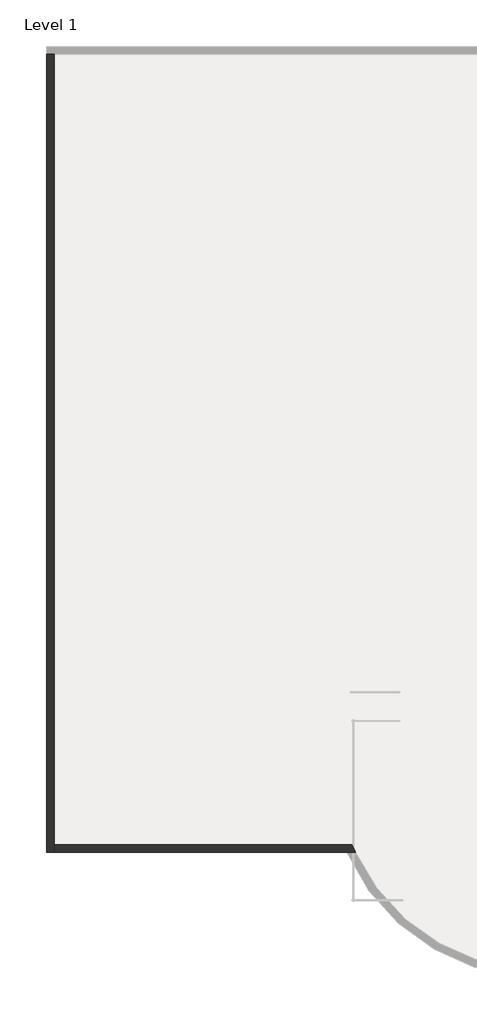
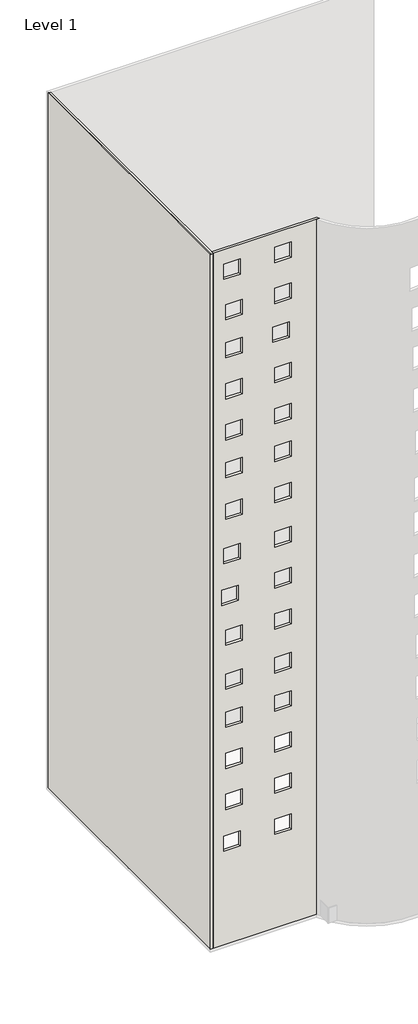
# One storey, part 1 of 3: 2 walls.
"""IFC4 building model written with IfcOpenShell, lengths in millimetres."""

from ifc_helpers import new_model, si_unit, frame, origin, place, context, project, spatial, polyline, circle_curve, faceted_brep, element, save
from ifc_brep_helpers import plane_surface, revolved_surface, advanced_brep

model = new_model("IFC4")

# Units and contexts
model_context = context("Model", 3, world=origin())
ifc_project = project(units=[si_unit("LENGTHUNIT", "METRE", prefix="MILLI")], contexts=[model_context])

# Site, building, storey
site = spatial("IfcSite", under=ifc_project)
building = spatial("IfcBuilding", under=site)
storey = spatial("IfcBuildingStorey", under=building, Name="Level 1", Elevation=0.0)

# Walls
placement = place(None, origin())
element("IfcWall", 1, ObjectType="Generic - 8\"", at=placement, inside=storey, context=model_context, shape_type="Brep", body=[
    faceted_brep([(-16607.9505427, 7156.3191779, 0.0), (-16607.9505427, -14078.0808221, 0.0), (-16607.9505427, -14078.0808221, 55473.6), (-16607.9505427, 7156.3191779, 55473.6), (-16404.7505427, 7156.3191779, 0.0), (-16404.7505427, 7156.3191779, 55473.6), (-16404.7505427, -13874.8808221, 55473.6), (-16404.7505427, -14078.0808221, 55473.6), (-16404.7505427, -14078.0808221, 0.0), (-16404.7505427, -13874.8808221, 0.0), (-16556.2150607, 7156.3191779, 55473.6), (-16556.2150607, -14078.0808221, 55473.6)], [[[0, 1, 2, 3]], [[4, 5, 6, 7, 8, 9]], [[1, 0, 4, 9, 8]], [[0, 3, 10, 5, 4]], [[2, 1, 8, 7, 11]], [[3, 2, 11, 10]], [[11, 7, 6, 5, 10]]]),
])
element("IfcWall", 2, ObjectType="Generic - 8\"", at=placement, inside=storey, context=model_context, shape_type="AdvancedBrep", body=[
    advanced_brep(
    [(-16404.7505427, -14078.0808221, 0.0), (-8605.1750786, -14078.0808221, 0.0), (-8381.8075047, -14078.0808221, 0.0), (-8381.8075047, -14078.0808221, 55473.6), (-8605.1750786, -14078.0808221, 55473.6), (-16404.7505427, -14078.0808221, 55473.6), (-15591.9505427, -14078.0808221, 54330.6), (-14372.7505427, -14078.0808221, 54330.6), (-14372.7505427, -14078.0808221, 53111.4), (-15591.9505427, -14078.0808221, 53111.4), (-11739.2382271, -14078.0808221, 54330.6), (-10520.0382271, -14078.0808221, 54330.6), (-10520.0382271, -14078.0808221, 53111.4), (-11739.2382271, -14078.0808221, 53111.4), (-15439.5505427, -14078.0808221, 51054.0), (-14220.3505427, -14078.0808221, 51054.0), (-14220.3505427, -14078.0808221, 49834.8), (-15439.5505427, -14078.0808221, 49834.8), (-11739.2382271, -14078.0808221, 51054.0), (-10520.0382271, -14078.0808221, 51054.0), (-10520.0382271, -14078.0808221, 49834.8), (-11739.2382271, -14078.0808221, 49834.8), (-15439.5505427, -14078.0808221, 48006.0), (-14220.3505427, -14078.0808221, 48006.0), (-14220.3505427, -14078.0808221, 46786.8), (-15439.5505427, -14078.0808221, 46786.8), (-11891.6382271, -14078.0808221, 48006.0), (-10672.4382271, -14078.0808221, 48006.0), (-10672.4382271, -14078.0808221, 46786.8), (-11891.6382271, -14078.0808221, 46786.8), (-15439.5505427, -14078.0808221, 44729.4), (-14220.3505427, -14078.0808221, 44729.4), (-14220.3505427, -14078.0808221, 43510.2), (-15439.5505427, -14078.0808221, 43510.2), (-11739.2382271, -14078.0808221, 44729.4), (-10520.0382271, -14078.0808221, 44729.4), (-10520.0382271, -14078.0808221, 43510.2), (-11739.2382271, -14078.0808221, 43510.2), (-15439.5505427, -14078.0808221, 41452.8), (-14220.3505427, -14078.0808221, 41452.8), (-14220.3505427, -14078.0808221, 40233.6), (-15439.5505427, -14078.0808221, 40233.6), (-11739.2382271, -14078.0808221, 41452.8), (-10520.0382271, -14078.0808221, 41452.8), (-10520.0382271, -14078.0808221, 40233.6), (-11739.2382271, -14078.0808221, 40233.6), (-15439.5505427, -14078.0808221, 38436.7791335), (-14220.3505427, -14078.0808221, 38436.7791335), (-14220.3505427, -14078.0808221, 37217.5791335), (-15439.5505427, -14078.0808221, 37217.5791335), (-11739.2382271, -14078.0808221, 38440.5564743), (-10520.0382271, -14078.0808221, 38440.5564743), (-10520.0382271, -14078.0808221, 37221.3564743), (-11739.2382271, -14078.0808221, 37221.3564743), (-15439.5505427, -14078.0808221, 35116.3338162), (-14220.3505427, -14078.0808221, 35116.3338162), (-14220.3505427, -14078.0808221, 33897.1338162), (-15439.5505427, -14078.0808221, 33897.1338162), (-11739.2382271, -14078.0808221, 35146.4998834), (-10520.0382271, -14078.0808221, 35146.4998834), (-10520.0382271, -14078.0808221, 33927.2998834), (-11739.2382271, -14078.0808221, 33927.2998834), (-15591.9505427, -14078.0808221, 31623.0), (-14372.7505427, -14078.0808221, 31623.0), (-14372.7505427, -14078.0808221, 30403.8), (-15591.9505427, -14078.0808221, 30403.8), (-11739.2382271, -14078.0808221, 31623.0), (-10520.0382271, -14078.0808221, 31623.0), (-10520.0382271, -14078.0808221, 30403.8), (-11739.2382271, -14078.0808221, 30403.8), (-15744.3505427, -14078.0808221, 28346.4), (-14525.1505427, -14078.0808221, 28346.4), (-14525.1505427, -14078.0808221, 27127.2), (-15744.3505427, -14078.0808221, 27127.2), (-11739.2382271, -14078.0808221, 28346.4), (-10520.0382271, -14078.0808221, 28346.4), (-10520.0382271, -14078.0808221, 27127.2), (-11739.2382271, -14078.0808221, 27127.2), (-15439.5505427, -14078.0808221, 25069.8), (-14220.3505427, -14078.0808221, 25069.8), (-14220.3505427, -14078.0808221, 23850.6), (-15439.5505427, -14078.0808221, 23850.6), (-11739.2382271, -14078.0808221, 25069.8), (-10520.0382271, -14078.0808221, 25069.8), (-10520.0382271, -14078.0808221, 23850.6), (-11739.2382271, -14078.0808221, 23850.6), (-15439.5505427, -14078.0808221, 21564.6), (-14220.3505427, -14078.0808221, 21564.6), (-14220.3505427, -14078.0808221, 20345.4), (-15439.5505427, -14078.0808221, 20345.4), (-11739.2382271, -14078.0808221, 21564.6), (-10520.0382271, -14078.0808221, 21564.6), (-10520.0382271, -14078.0808221, 20345.4), (-11739.2382271, -14078.0808221, 20345.4), (-11739.2382271, -14078.0808221, 18516.6), (-10520.0382271, -14078.0808221, 18516.6), (-10520.0382271, -14078.0808221, 17297.4), (-11739.2382271, -14078.0808221, 17297.4), (-15439.5505427, -14078.0808221, 18516.6), (-14220.3505427, -14078.0808221, 18516.6), (-14220.3505427, -14078.0808221, 17297.4), (-15439.5505427, -14078.0808221, 17297.4), (-11739.2382271, -14078.0808221, 15240.0), (-10520.0382271, -14078.0808221, 15240.0), (-10520.0382271, -14078.0808221, 14020.8), (-11739.2382271, -14078.0808221, 14020.8), (-15439.5505427, -14078.0808221, 15240.0), (-14220.3505427, -14078.0808221, 15240.0), (-14220.3505427, -14078.0808221, 14020.8), (-15439.5505427, -14078.0808221, 14020.8), (-11739.2382271, -14078.0808221, 11963.4), (-10520.0382271, -14078.0808221, 11963.4), (-10520.0382271, -14078.0808221, 10744.2), (-11739.2382271, -14078.0808221, 10744.2), (-15439.5505427, -14078.0808221, 11963.4), (-14220.3505427, -14078.0808221, 11963.4), (-14220.3505427, -14078.0808221, 10744.2), (-15439.5505427, -14078.0808221, 10744.2), (-15591.9505427, -14078.0808221, 8686.8), (-14372.7505427, -14078.0808221, 8686.8), (-14372.7505427, -14078.0808221, 7467.6), (-15591.9505427, -14078.0808221, 7467.6), (-11739.2382271, -14078.0808221, 8686.8), (-10520.0382271, -14078.0808221, 8686.8), (-10520.0382271, -14078.0808221, 7467.6), (-11739.2382271, -14078.0808221, 7467.6), (-16404.7505427, -13874.8808221, 0.0), (-16404.7505427, -13874.8808221, 55473.6), (-8471.6205396, -13874.8808221, 55473.6), (-8471.6205396, -13874.8808221, 0.0), (-15591.9505427, -13874.8808221, 54330.6), (-15591.9505427, -13874.8808221, 53111.4), (-14372.7505427, -13874.8808221, 53111.4), (-14372.7505427, -13874.8808221, 54330.6), (-11739.2382271, -13874.8808221, 54330.6), (-11739.2382271, -13874.8808221, 53111.4), (-10520.0382271, -13874.8808221, 53111.4), (-10520.0382271, -13874.8808221, 54330.6), (-15439.5505427, -13874.8808221, 51054.0), (-15439.5505427, -13874.8808221, 49834.8), (-14220.3505427, -13874.8808221, 49834.8), (-14220.3505427, -13874.8808221, 51054.0), (-11739.2382271, -13874.8808221, 51054.0), (-11739.2382271, -13874.8808221, 49834.8), (-10520.0382271, -13874.8808221, 49834.8), (-10520.0382271, -13874.8808221, 51054.0), (-15439.5505427, -13874.8808221, 48006.0), (-15439.5505427, -13874.8808221, 46786.8), (-14220.3505427, -13874.8808221, 46786.8), (-14220.3505427, -13874.8808221, 48006.0), (-11891.6382271, -13874.8808221, 48006.0), (-11891.6382271, -13874.8808221, 46786.8), (-10672.4382271, -13874.8808221, 46786.8), (-10672.4382271, -13874.8808221, 48006.0), (-15439.5505427, -13874.8808221, 44729.4), (-15439.5505427, -13874.8808221, 43510.2), (-14220.3505427, -13874.8808221, 43510.2), (-14220.3505427, -13874.8808221, 44729.4), (-11739.2382271, -13874.8808221, 44729.4), (-11739.2382271, -13874.8808221, 43510.2), (-10520.0382271, -13874.8808221, 43510.2), (-10520.0382271, -13874.8808221, 44729.4), (-15439.5505427, -13874.8808221, 41452.8), (-15439.5505427, -13874.8808221, 40233.6), (-14220.3505427, -13874.8808221, 40233.6), (-14220.3505427, -13874.8808221, 41452.8), (-11739.2382271, -13874.8808221, 41452.8), (-11739.2382271, -13874.8808221, 40233.6), (-10520.0382271, -13874.8808221, 40233.6), (-10520.0382271, -13874.8808221, 41452.8), (-15439.5505427, -13874.8808221, 38436.7791335), (-15439.5505427, -13874.8808221, 37217.5791335), (-14220.3505427, -13874.8808221, 37217.5791335), (-14220.3505427, -13874.8808221, 38436.7791335), (-11739.2382271, -13874.8808221, 38440.5564743), (-11739.2382271, -13874.8808221, 37221.3564743), (-10520.0382271, -13874.8808221, 37221.3564743), (-10520.0382271, -13874.8808221, 38440.5564743), (-15439.5505427, -13874.8808221, 35116.3338162), (-15439.5505427, -13874.8808221, 33897.1338162), (-14220.3505427, -13874.8808221, 33897.1338162), (-14220.3505427, -13874.8808221, 35116.3338162), (-11739.2382271, -13874.8808221, 35146.4998834), (-11739.2382271, -13874.8808221, 33927.2998834), (-10520.0382271, -13874.8808221, 33927.2998834), (-10520.0382271, -13874.8808221, 35146.4998834), (-15591.9505427, -13874.8808221, 31623.0), (-15591.9505427, -13874.8808221, 30403.8), (-14372.7505427, -13874.8808221, 30403.8), (-14372.7505427, -13874.8808221, 31623.0), (-11739.2382271, -13874.8808221, 31623.0), (-11739.2382271, -13874.8808221, 30403.8), (-10520.0382271, -13874.8808221, 30403.8), (-10520.0382271, -13874.8808221, 31623.0), (-15744.3505427, -13874.8808221, 28346.4), (-15744.3505427, -13874.8808221, 27127.2), (-14525.1505427, -13874.8808221, 27127.2), (-14525.1505427, -13874.8808221, 28346.4), (-11739.2382271, -13874.8808221, 28346.4), (-11739.2382271, -13874.8808221, 27127.2), (-10520.0382271, -13874.8808221, 27127.2), (-10520.0382271, -13874.8808221, 28346.4), (-15439.5505427, -13874.8808221, 25069.8), (-15439.5505427, -13874.8808221, 23850.6), (-14220.3505427, -13874.8808221, 23850.6), (-14220.3505427, -13874.8808221, 25069.8), (-11739.2382271, -13874.8808221, 25069.8), (-11739.2382271, -13874.8808221, 23850.6), (-10520.0382271, -13874.8808221, 23850.6), (-10520.0382271, -13874.8808221, 25069.8), (-15439.5505427, -13874.8808221, 21564.6), (-15439.5505427, -13874.8808221, 20345.4), (-14220.3505427, -13874.8808221, 20345.4), (-14220.3505427, -13874.8808221, 21564.6), (-11739.2382271, -13874.8808221, 21564.6), (-11739.2382271, -13874.8808221, 20345.4), (-10520.0382271, -13874.8808221, 20345.4), (-10520.0382271, -13874.8808221, 21564.6), (-11739.2382271, -13874.8808221, 18516.6), (-11739.2382271, -13874.8808221, 17297.4), (-10520.0382271, -13874.8808221, 17297.4), (-10520.0382271, -13874.8808221, 18516.6), (-15439.5505427, -13874.8808221, 18516.6), (-15439.5505427, -13874.8808221, 17297.4), (-14220.3505427, -13874.8808221, 17297.4), (-14220.3505427, -13874.8808221, 18516.6), (-11739.2382271, -13874.8808221, 15240.0), (-11739.2382271, -13874.8808221, 14020.8), (-10520.0382271, -13874.8808221, 14020.8), (-10520.0382271, -13874.8808221, 15240.0), (-15439.5505427, -13874.8808221, 15240.0), (-15439.5505427, -13874.8808221, 14020.8), (-14220.3505427, -13874.8808221, 14020.8), (-14220.3505427, -13874.8808221, 15240.0), (-11739.2382271, -13874.8808221, 11963.4), (-11739.2382271, -13874.8808221, 10744.2), (-10520.0382271, -13874.8808221, 10744.2), (-10520.0382271, -13874.8808221, 11963.4), (-15439.5505427, -13874.8808221, 11963.4), (-15439.5505427, -13874.8808221, 10744.2), (-14220.3505427, -13874.8808221, 10744.2), (-14220.3505427, -13874.8808221, 11963.4), (-15591.9505427, -13874.8808221, 8686.8), (-15591.9505427, -13874.8808221, 7467.6), (-14372.7505427, -13874.8808221, 7467.6), (-14372.7505427, -13874.8808221, 8686.8), (-11739.2382271, -13874.8808221, 8686.8), (-11739.2382271, -13874.8808221, 7467.6), (-10520.0382271, -13874.8808221, 7467.6), (-10520.0382271, -13874.8808221, 8686.8)],
    [
        (0, 1),
        (1, 2),
        (2, 3),
        (3, 4),
        (4, 5),
        (5, 0),
        (6, 7),
        (7, 8),
        (8, 9),
        (9, 6),
        (10, 11),
        (11, 12),
        (12, 13),
        (13, 10),
        (14, 15),
        (15, 16),
        (16, 17),
        (17, 14),
        (18, 19),
        (19, 20),
        (20, 21),
        (21, 18),
        (22, 23),
        (23, 24),
        (24, 25),
        (25, 22),
        (26, 27),
        (27, 28),
        (28, 29),
        (29, 26),
        (30, 31),
        (31, 32),
        (32, 33),
        (33, 30),
        (34, 35),
        (35, 36),
        (36, 37),
        (37, 34),
        (38, 39),
        (39, 40),
        (40, 41),
        (41, 38),
        (42, 43),
        (43, 44),
        (44, 45),
        (45, 42),
        (46, 47),
        (47, 48),
        (48, 49),
        (49, 46),
        (50, 51),
        (51, 52),
        (52, 53),
        (53, 50),
        (54, 55),
        (55, 56),
        (56, 57),
        (57, 54),
        (58, 59),
        (59, 60),
        (60, 61),
        (61, 58),
        (62, 63),
        (63, 64),
        (64, 65),
        (65, 62),
        (66, 67),
        (67, 68),
        (68, 69),
        (69, 66),
        (70, 71),
        (71, 72),
        (72, 73),
        (73, 70),
        (74, 75),
        (75, 76),
        (76, 77),
        (77, 74),
        (78, 79),
        (79, 80),
        (80, 81),
        (81, 78),
        (82, 83),
        (83, 84),
        (84, 85),
        (85, 82),
        (86, 87),
        (87, 88),
        (88, 89),
        (89, 86),
        (90, 91),
        (91, 92),
        (92, 93),
        (93, 90),
        (94, 95),
        (95, 96),
        (96, 97),
        (97, 94),
        (98, 99),
        (99, 100),
        (100, 101),
        (101, 98),
        (102, 103),
        (103, 104),
        (104, 105),
        (105, 102),
        (106, 107),
        (107, 108),
        (108, 109),
        (109, 106),
        (110, 111),
        (111, 112),
        (112, 113),
        (113, 110),
        (114, 115),
        (115, 116),
        (116, 117),
        (117, 114),
        (118, 119),
        (119, 120),
        (120, 121),
        (121, 118),
        (122, 123),
        (123, 124),
        (124, 125),
        (125, 122),
        (126, 127),
        (127, 128),
        (128, 129),
        (129, 126),
        (130, 131),
        (131, 132),
        (132, 133),
        (133, 130),
        (134, 135),
        (135, 136),
        (136, 137),
        (137, 134),
        (138, 139),
        (139, 140),
        (140, 141),
        (141, 138),
        (142, 143),
        (143, 144),
        (144, 145),
        (145, 142),
        (146, 147),
        (147, 148),
        (148, 149),
        (149, 146),
        (150, 151),
        (151, 152),
        (152, 153),
        (153, 150),
        (154, 155),
        (155, 156),
        (156, 157),
        (157, 154),
        (158, 159),
        (159, 160),
        (160, 161),
        (161, 158),
        (162, 163),
        (163, 164),
        (164, 165),
        (165, 162),
        (166, 167),
        (167, 168),
        (168, 169),
        (169, 166),
        (170, 171),
        (171, 172),
        (172, 173),
        (173, 170),
        (174, 175),
        (175, 176),
        (176, 177),
        (177, 174),
        (178, 179),
        (179, 180),
        (180, 181),
        (181, 178),
        (182, 183),
        (183, 184),
        (184, 185),
        (185, 182),
        (186, 187),
        (187, 188),
        (188, 189),
        (189, 186),
        (190, 191),
        (191, 192),
        (192, 193),
        (193, 190),
        (194, 195),
        (195, 196),
        (196, 197),
        (197, 194),
        (198, 199),
        (199, 200),
        (200, 201),
        (201, 198),
        (202, 203),
        (203, 204),
        (204, 205),
        (205, 202),
        (206, 207),
        (207, 208),
        (208, 209),
        (209, 206),
        (210, 211),
        (211, 212),
        (212, 213),
        (213, 210),
        (214, 215),
        (215, 216),
        (216, 217),
        (217, 214),
        (218, 219),
        (219, 220),
        (220, 221),
        (221, 218),
        (222, 223),
        (223, 224),
        (224, 225),
        (225, 222),
        (226, 227),
        (227, 228),
        (228, 229),
        (229, 226),
        (230, 231),
        (231, 232),
        (232, 233),
        (233, 230),
        (234, 235),
        (235, 236),
        (236, 237),
        (237, 234),
        (238, 239),
        (239, 240),
        (240, 241),
        (241, 238),
        (242, 243),
        (243, 244),
        (244, 245),
        (245, 242),
        (246, 247),
        (247, 248),
        (248, 249),
        (249, 246),
        (0, 126),
        (129, 2, circle_curve(frame((-3476.1505427, -11788.3650223, 0.0), z_axis=(0.0, 0.0, 1.0), x_axis=(1.0, 0.0, 0.0)), 5413.7111737)),
        (5, 127),
        (128, 3, circle_curve(frame((-3476.1505427, -11788.3650223, 55473.6), z_axis=(0.0, 0.0, 1.0), x_axis=(1.0, 0.0, 0.0)), 5413.7111737)),
        (130, 6),
        (9, 131),
        (8, 132),
        (7, 133),
        (134, 10),
        (13, 135),
        (12, 136),
        (11, 137),
        (138, 14),
        (17, 139),
        (16, 140),
        (15, 141),
        (142, 18),
        (21, 143),
        (20, 144),
        (19, 145),
        (146, 22),
        (25, 147),
        (24, 148),
        (23, 149),
        (150, 26),
        (29, 151),
        (28, 152),
        (27, 153),
        (154, 30),
        (33, 155),
        (32, 156),
        (31, 157),
        (158, 34),
        (37, 159),
        (36, 160),
        (35, 161),
        (162, 38),
        (41, 163),
        (40, 164),
        (39, 165),
        (166, 42),
        (45, 167),
        (44, 168),
        (43, 169),
        (170, 46),
        (49, 171),
        (48, 172),
        (47, 173),
        (174, 50),
        (53, 175),
        (52, 176),
        (51, 177),
        (178, 54),
        (57, 179),
        (56, 180),
        (55, 181),
        (182, 58),
        (61, 183),
        (60, 184),
        (59, 185),
        (186, 62),
        (65, 187),
        (64, 188),
        (63, 189),
        (190, 66),
        (69, 191),
        (68, 192),
        (67, 193),
        (194, 70),
        (73, 195),
        (72, 196),
        (71, 197),
        (198, 74),
        (77, 199),
        (76, 200),
        (75, 201),
        (202, 78),
        (81, 203),
        (80, 204),
        (79, 205),
        (206, 82),
        (85, 207),
        (84, 208),
        (83, 209),
        (210, 86),
        (89, 211),
        (88, 212),
        (87, 213),
        (214, 90),
        (93, 215),
        (92, 216),
        (91, 217),
        (218, 94),
        (97, 219),
        (96, 220),
        (95, 221),
        (222, 98),
        (101, 223),
        (100, 224),
        (99, 225),
        (226, 102),
        (105, 227),
        (104, 228),
        (103, 229),
        (230, 106),
        (109, 231),
        (108, 232),
        (107, 233),
        (234, 110),
        (113, 235),
        (112, 236),
        (111, 237),
        (238, 114),
        (117, 239),
        (116, 240),
        (115, 241),
        (242, 118),
        (121, 243),
        (120, 244),
        (119, 245),
        (246, 122),
        (125, 247),
        (124, 248),
        (123, 249),
    ],
    [
        plane_surface(frame((-16506.3505427, -14078.0808221, 0.0), z_axis=(0.0, -1.0, 0.0), x_axis=(1.0, 0.0, 0.0))),
        plane_surface(frame((-16506.3505427, -13874.8808221, 0.0), z_axis=(0.0, 1.0, 0.0), x_axis=(-1.0, 0.0, 0.0))),
        plane_surface(frame((-16506.3505427, -14078.0808221, 0.0), z_axis=(0.0, 0.0, -1.0), x_axis=(0.0, 1.0, 0.0))),
        plane_surface(frame((-16404.7505427, 7359.5191779, 0.0), z_axis=(-1.0, 0.0, 0.0), x_axis=(0.0, 1.0, 0.0))),
        revolved_surface(polyline([(1937.5606309999994, -11788.3650223, 0.0), (1937.5606309999994, -11788.3650223, 55473.6)]), (-3476.1505427, -11788.3650223, 0.0), (0.0, 0.0, -1.0)),
        plane_surface(frame((-15591.9505427, -13874.8808221, 54330.6), z_axis=(1.0, 0.0, 0.0), x_axis=(0.0, -1.0, 0.0))),
        plane_surface(frame((-15591.9505427, -13874.8808221, 53111.4), z_axis=(0.0, 0.0, 1.0), x_axis=(0.0, -1.0, 0.0))),
        plane_surface(frame((-14372.7505427, -13874.8808221, 53111.4), z_axis=(-1.0, 0.0, 0.0), x_axis=(0.0, -1.0, 0.0))),
        plane_surface(frame((-14372.7505427, -13874.8808221, 54330.6), z_axis=(0.0, 0.0, -1.0), x_axis=(0.0, -1.0, 0.0))),
        plane_surface(frame((-11739.2382271, -13874.8808221, 54330.6), z_axis=(1.0, 0.0, 0.0), x_axis=(0.0, -1.0, 0.0))),
        plane_surface(frame((-11739.2382271, -13874.8808221, 53111.4), z_axis=(0.0, 0.0, 1.0), x_axis=(0.0, -1.0, 0.0))),
        plane_surface(frame((-10520.0382271, -13874.8808221, 53111.4), z_axis=(-1.0, 0.0, 0.0), x_axis=(0.0, -1.0, 0.0))),
        plane_surface(frame((-10520.0382271, -13874.8808221, 54330.6), z_axis=(0.0, 0.0, -1.0), x_axis=(0.0, -1.0, 0.0))),
        plane_surface(frame((-15439.5505427, -13874.8808221, 51054.0), z_axis=(1.0, 0.0, 0.0), x_axis=(0.0, -1.0, 0.0))),
        plane_surface(frame((-15439.5505427, -13874.8808221, 49834.8), z_axis=(0.0, 0.0, 1.0), x_axis=(0.0, -1.0, 0.0))),
        plane_surface(frame((-14220.3505427, -13874.8808221, 49834.8), z_axis=(-1.0, 0.0, 0.0), x_axis=(0.0, -1.0, 0.0))),
        plane_surface(frame((-14220.3505427, -13874.8808221, 51054.0), z_axis=(0.0, 0.0, -1.0), x_axis=(0.0, -1.0, 0.0))),
        plane_surface(frame((-11739.2382271, -13874.8808221, 51054.0), z_axis=(1.0, 0.0, 0.0), x_axis=(0.0, -1.0, 0.0))),
        plane_surface(frame((-11739.2382271, -13874.8808221, 49834.8), z_axis=(0.0, 0.0, 1.0), x_axis=(0.0, -1.0, 0.0))),
        plane_surface(frame((-10520.0382271, -13874.8808221, 49834.8), z_axis=(-1.0, 0.0, 0.0), x_axis=(0.0, -1.0, 0.0))),
        plane_surface(frame((-10520.0382271, -13874.8808221, 51054.0), z_axis=(0.0, 0.0, -1.0), x_axis=(0.0, -1.0, 0.0))),
        plane_surface(frame((-15439.5505427, -13874.8808221, 48006.0), z_axis=(1.0, 0.0, 0.0), x_axis=(0.0, -1.0, 0.0))),
        plane_surface(frame((-15439.5505427, -13874.8808221, 46786.8), z_axis=(0.0, 0.0, 1.0), x_axis=(0.0, -1.0, 0.0))),
        plane_surface(frame((-14220.3505427, -13874.8808221, 46786.8), z_axis=(-1.0, 0.0, 0.0), x_axis=(0.0, -1.0, 0.0))),
        plane_surface(frame((-14220.3505427, -13874.8808221, 48006.0), z_axis=(0.0, 0.0, -1.0), x_axis=(0.0, -1.0, 0.0))),
        plane_surface(frame((-11891.6382271, -13874.8808221, 48006.0), z_axis=(1.0, 0.0, 0.0), x_axis=(0.0, -1.0, 0.0))),
        plane_surface(frame((-11891.6382271, -13874.8808221, 46786.8), z_axis=(0.0, 0.0, 1.0), x_axis=(0.0, -1.0, 0.0))),
        plane_surface(frame((-10672.4382271, -13874.8808221, 46786.8), z_axis=(-1.0, 0.0, 0.0), x_axis=(0.0, -1.0, 0.0))),
        plane_surface(frame((-10672.4382271, -13874.8808221, 48006.0), z_axis=(0.0, 0.0, -1.0), x_axis=(0.0, -1.0, 0.0))),
        plane_surface(frame((-15439.5505427, -13874.8808221, 44729.4), z_axis=(1.0, 0.0, 0.0), x_axis=(0.0, -1.0, 0.0))),
        plane_surface(frame((-15439.5505427, -13874.8808221, 43510.2), z_axis=(0.0, 0.0, 1.0), x_axis=(0.0, -1.0, 0.0))),
        plane_surface(frame((-14220.3505427, -13874.8808221, 43510.2), z_axis=(-1.0, 0.0, 0.0), x_axis=(0.0, -1.0, 0.0))),
        plane_surface(frame((-14220.3505427, -13874.8808221, 44729.4), z_axis=(0.0, 0.0, -1.0), x_axis=(0.0, -1.0, 0.0))),
        plane_surface(frame((-11739.2382271, -13874.8808221, 44729.4), z_axis=(1.0, 0.0, 0.0), x_axis=(0.0, -1.0, 0.0))),
        plane_surface(frame((-11739.2382271, -13874.8808221, 43510.2), z_axis=(0.0, 0.0, 1.0), x_axis=(0.0, -1.0, 0.0))),
        plane_surface(frame((-10520.0382271, -13874.8808221, 43510.2), z_axis=(-1.0, 0.0, 0.0), x_axis=(0.0, -1.0, 0.0))),
        plane_surface(frame((-10520.0382271, -13874.8808221, 44729.4), z_axis=(0.0, 0.0, -1.0), x_axis=(0.0, -1.0, 0.0))),
        plane_surface(frame((-15439.5505427, -13874.8808221, 41452.8), z_axis=(1.0, 0.0, 0.0), x_axis=(0.0, -1.0, 0.0))),
        plane_surface(frame((-15439.5505427, -13874.8808221, 40233.6), z_axis=(0.0, 0.0, 1.0), x_axis=(0.0, -1.0, 0.0))),
        plane_surface(frame((-14220.3505427, -13874.8808221, 40233.6), z_axis=(-1.0, 0.0, 0.0), x_axis=(0.0, -1.0, 0.0))),
        plane_surface(frame((-14220.3505427, -13874.8808221, 41452.8), z_axis=(0.0, 0.0, -1.0), x_axis=(0.0, -1.0, 0.0))),
        plane_surface(frame((-11739.2382271, -13874.8808221, 41452.8), z_axis=(1.0, 0.0, 0.0), x_axis=(0.0, -1.0, 0.0))),
        plane_surface(frame((-11739.2382271, -13874.8808221, 40233.6), z_axis=(0.0, 0.0, 1.0), x_axis=(0.0, -1.0, 0.0))),
        plane_surface(frame((-10520.0382271, -13874.8808221, 40233.6), z_axis=(-1.0, 0.0, 0.0), x_axis=(0.0, -1.0, 0.0))),
        plane_surface(frame((-10520.0382271, -13874.8808221, 41452.8), z_axis=(0.0, 0.0, -1.0), x_axis=(0.0, -1.0, 0.0))),
        plane_surface(frame((-15439.5505427, -13874.8808221, 38436.7791335), z_axis=(1.0, 0.0, 0.0), x_axis=(0.0, -1.0, 0.0))),
        plane_surface(frame((-15439.5505427, -13874.8808221, 37217.5791335), z_axis=(0.0, 0.0, 1.0), x_axis=(0.0, -1.0, 0.0))),
        plane_surface(frame((-14220.3505427, -13874.8808221, 37217.5791335), z_axis=(-1.0, 0.0, 0.0), x_axis=(0.0, -1.0, 0.0))),
        plane_surface(frame((-14220.3505427, -13874.8808221, 38436.7791335), z_axis=(0.0, 0.0, -1.0), x_axis=(0.0, -1.0, 0.0))),
        plane_surface(frame((-11739.2382271, -13874.8808221, 38440.5564743), z_axis=(1.0, 0.0, 0.0), x_axis=(0.0, -1.0, 0.0))),
        plane_surface(frame((-11739.2382271, -13874.8808221, 37221.3564743), z_axis=(0.0, 0.0, 1.0), x_axis=(0.0, -1.0, 0.0))),
        plane_surface(frame((-10520.0382271, -13874.8808221, 37221.3564743), z_axis=(-1.0, 0.0, 0.0), x_axis=(0.0, -1.0, 0.0))),
        plane_surface(frame((-10520.0382271, -13874.8808221, 38440.5564743), z_axis=(0.0, 0.0, -1.0), x_axis=(0.0, -1.0, 0.0))),
        plane_surface(frame((-15439.5505427, -13874.8808221, 35116.3338162), z_axis=(1.0, 0.0, 0.0), x_axis=(0.0, -1.0, 0.0))),
        plane_surface(frame((-15439.5505427, -13874.8808221, 33897.1338162), z_axis=(0.0, 0.0, 1.0), x_axis=(0.0, -1.0, 0.0))),
        plane_surface(frame((-14220.3505427, -13874.8808221, 33897.1338162), z_axis=(-1.0, 0.0, 0.0), x_axis=(0.0, -1.0, 0.0))),
        plane_surface(frame((-14220.3505427, -13874.8808221, 35116.3338162), z_axis=(0.0, 0.0, -1.0), x_axis=(0.0, -1.0, 0.0))),
        plane_surface(frame((-11739.2382271, -13874.8808221, 35146.4998834), z_axis=(1.0, 0.0, 0.0), x_axis=(0.0, -1.0, 0.0))),
        plane_surface(frame((-11739.2382271, -13874.8808221, 33927.2998834), z_axis=(0.0, 0.0, 1.0), x_axis=(0.0, -1.0, 0.0))),
        plane_surface(frame((-10520.0382271, -13874.8808221, 33927.2998834), z_axis=(-1.0, 0.0, 0.0), x_axis=(0.0, -1.0, 0.0))),
        plane_surface(frame((-10520.0382271, -13874.8808221, 35146.4998834), z_axis=(0.0, 0.0, -1.0), x_axis=(0.0, -1.0, 0.0))),
        plane_surface(frame((-15591.9505427, -13874.8808221, 31623.0), z_axis=(1.0, 0.0, 0.0), x_axis=(0.0, -1.0, 0.0))),
        plane_surface(frame((-15591.9505427, -13874.8808221, 30403.8), z_axis=(0.0, 0.0, 1.0), x_axis=(0.0, -1.0, 0.0))),
        plane_surface(frame((-14372.7505427, -13874.8808221, 30403.8), z_axis=(-1.0, 0.0, 0.0), x_axis=(0.0, -1.0, 0.0))),
        plane_surface(frame((-14372.7505427, -13874.8808221, 31623.0), z_axis=(0.0, 0.0, -1.0), x_axis=(0.0, -1.0, 0.0))),
        plane_surface(frame((-11739.2382271, -13874.8808221, 31623.0), z_axis=(1.0, 0.0, 0.0), x_axis=(0.0, -1.0, 0.0))),
        plane_surface(frame((-11739.2382271, -13874.8808221, 30403.8), z_axis=(0.0, 0.0, 1.0), x_axis=(0.0, -1.0, 0.0))),
        plane_surface(frame((-10520.0382271, -13874.8808221, 30403.8), z_axis=(-1.0, 0.0, 0.0), x_axis=(0.0, -1.0, 0.0))),
        plane_surface(frame((-10520.0382271, -13874.8808221, 31623.0), z_axis=(0.0, 0.0, -1.0), x_axis=(0.0, -1.0, 0.0))),
        plane_surface(frame((-15744.3505427, -13874.8808221, 28346.4), z_axis=(1.0, 0.0, 0.0), x_axis=(0.0, -1.0, 0.0))),
        plane_surface(frame((-15744.3505427, -13874.8808221, 27127.2), z_axis=(0.0, 0.0, 1.0), x_axis=(0.0, -1.0, 0.0))),
        plane_surface(frame((-14525.1505427, -13874.8808221, 27127.2), z_axis=(-1.0, 0.0, 0.0), x_axis=(0.0, -1.0, 0.0))),
        plane_surface(frame((-14525.1505427, -13874.8808221, 28346.4), z_axis=(0.0, 0.0, -1.0), x_axis=(0.0, -1.0, 0.0))),
        plane_surface(frame((-11739.2382271, -13874.8808221, 28346.4), z_axis=(1.0, 0.0, 0.0), x_axis=(0.0, -1.0, 0.0))),
        plane_surface(frame((-11739.2382271, -13874.8808221, 27127.2), z_axis=(0.0, 0.0, 1.0), x_axis=(0.0, -1.0, 0.0))),
        plane_surface(frame((-10520.0382271, -13874.8808221, 27127.2), z_axis=(-1.0, 0.0, 0.0), x_axis=(0.0, -1.0, 0.0))),
        plane_surface(frame((-10520.0382271, -13874.8808221, 28346.4), z_axis=(0.0, 0.0, -1.0), x_axis=(0.0, -1.0, 0.0))),
        plane_surface(frame((-15439.5505427, -13874.8808221, 25069.8), z_axis=(1.0, 0.0, 0.0), x_axis=(0.0, -1.0, 0.0))),
        plane_surface(frame((-15439.5505427, -13874.8808221, 23850.6), z_axis=(0.0, 0.0, 1.0), x_axis=(0.0, -1.0, 0.0))),
        plane_surface(frame((-14220.3505427, -13874.8808221, 23850.6), z_axis=(-1.0, 0.0, 0.0), x_axis=(0.0, -1.0, 0.0))),
        plane_surface(frame((-14220.3505427, -13874.8808221, 25069.8), z_axis=(0.0, 0.0, -1.0), x_axis=(0.0, -1.0, 0.0))),
        plane_surface(frame((-11739.2382271, -13874.8808221, 25069.8), z_axis=(1.0, 0.0, 0.0), x_axis=(0.0, -1.0, 0.0))),
        plane_surface(frame((-11739.2382271, -13874.8808221, 23850.6), z_axis=(0.0, 0.0, 1.0), x_axis=(0.0, -1.0, 0.0))),
        plane_surface(frame((-10520.0382271, -13874.8808221, 23850.6), z_axis=(-1.0, 0.0, 0.0), x_axis=(0.0, -1.0, 0.0))),
        plane_surface(frame((-10520.0382271, -13874.8808221, 25069.8), z_axis=(0.0, 0.0, -1.0), x_axis=(0.0, -1.0, 0.0))),
        plane_surface(frame((-15439.5505427, -13874.8808221, 21564.6), z_axis=(1.0, 0.0, 0.0), x_axis=(0.0, -1.0, 0.0))),
        plane_surface(frame((-15439.5505427, -13874.8808221, 20345.4), z_axis=(0.0, 0.0, 1.0), x_axis=(0.0, -1.0, 0.0))),
        plane_surface(frame((-14220.3505427, -13874.8808221, 20345.4), z_axis=(-1.0, 0.0, 0.0), x_axis=(0.0, -1.0, 0.0))),
        plane_surface(frame((-14220.3505427, -13874.8808221, 21564.6), z_axis=(0.0, 0.0, -1.0), x_axis=(0.0, -1.0, 0.0))),
        plane_surface(frame((-11739.2382271, -13874.8808221, 21564.6), z_axis=(1.0, 0.0, 0.0), x_axis=(0.0, -1.0, 0.0))),
        plane_surface(frame((-11739.2382271, -13874.8808221, 20345.4), z_axis=(0.0, 0.0, 1.0), x_axis=(0.0, -1.0, 0.0))),
        plane_surface(frame((-10520.0382271, -13874.8808221, 20345.4), z_axis=(-1.0, 0.0, 0.0), x_axis=(0.0, -1.0, 0.0))),
        plane_surface(frame((-10520.0382271, -13874.8808221, 21564.6), z_axis=(0.0, 0.0, -1.0), x_axis=(0.0, -1.0, 0.0))),
        plane_surface(frame((-11739.2382271, -13874.8808221, 18516.6), z_axis=(1.0, 0.0, 0.0), x_axis=(0.0, -1.0, 0.0))),
        plane_surface(frame((-11739.2382271, -13874.8808221, 17297.4), z_axis=(0.0, 0.0, 1.0), x_axis=(0.0, -1.0, 0.0))),
        plane_surface(frame((-10520.0382271, -13874.8808221, 17297.4), z_axis=(-1.0, 0.0, 0.0), x_axis=(0.0, -1.0, 0.0))),
        plane_surface(frame((-10520.0382271, -13874.8808221, 18516.6), z_axis=(0.0, 0.0, -1.0), x_axis=(0.0, -1.0, 0.0))),
        plane_surface(frame((-15439.5505427, -13874.8808221, 18516.6), z_axis=(1.0, 0.0, 0.0), x_axis=(0.0, -1.0, 0.0))),
        plane_surface(frame((-15439.5505427, -13874.8808221, 17297.4), z_axis=(0.0, 0.0, 1.0), x_axis=(0.0, -1.0, 0.0))),
        plane_surface(frame((-14220.3505427, -13874.8808221, 17297.4), z_axis=(-1.0, 0.0, 0.0), x_axis=(0.0, -1.0, 0.0))),
        plane_surface(frame((-14220.3505427, -13874.8808221, 18516.6), z_axis=(0.0, 0.0, -1.0), x_axis=(0.0, -1.0, 0.0))),
        plane_surface(frame((-11739.2382271, -13874.8808221, 15240.0), z_axis=(1.0, 0.0, 0.0), x_axis=(0.0, -1.0, 0.0))),
        plane_surface(frame((-11739.2382271, -13874.8808221, 14020.8), z_axis=(0.0, 0.0, 1.0), x_axis=(0.0, -1.0, 0.0))),
        plane_surface(frame((-10520.0382271, -13874.8808221, 14020.8), z_axis=(-1.0, 0.0, 0.0), x_axis=(0.0, -1.0, 0.0))),
        plane_surface(frame((-10520.0382271, -13874.8808221, 15240.0), z_axis=(0.0, 0.0, -1.0), x_axis=(0.0, -1.0, 0.0))),
        plane_surface(frame((-15439.5505427, -13874.8808221, 15240.0), z_axis=(1.0, 0.0, 0.0), x_axis=(0.0, -1.0, 0.0))),
        plane_surface(frame((-15439.5505427, -13874.8808221, 14020.8), z_axis=(0.0, 0.0, 1.0), x_axis=(0.0, -1.0, 0.0))),
        plane_surface(frame((-14220.3505427, -13874.8808221, 14020.8), z_axis=(-1.0, 0.0, 0.0), x_axis=(0.0, -1.0, 0.0))),
        plane_surface(frame((-14220.3505427, -13874.8808221, 15240.0), z_axis=(0.0, 0.0, -1.0), x_axis=(0.0, -1.0, 0.0))),
        plane_surface(frame((-11739.2382271, -13874.8808221, 11963.4), z_axis=(1.0, 0.0, 0.0), x_axis=(0.0, -1.0, 0.0))),
        plane_surface(frame((-11739.2382271, -13874.8808221, 10744.2), z_axis=(0.0, 0.0, 1.0), x_axis=(0.0, -1.0, 0.0))),
        plane_surface(frame((-10520.0382271, -13874.8808221, 10744.2), z_axis=(-1.0, 0.0, 0.0), x_axis=(0.0, -1.0, 0.0))),
        plane_surface(frame((-10520.0382271, -13874.8808221, 11963.4), z_axis=(0.0, 0.0, -1.0), x_axis=(0.0, -1.0, 0.0))),
        plane_surface(frame((-15439.5505427, -13874.8808221, 11963.4), z_axis=(1.0, 0.0, 0.0), x_axis=(0.0, -1.0, 0.0))),
        plane_surface(frame((-15439.5505427, -13874.8808221, 10744.2), z_axis=(0.0, 0.0, 1.0), x_axis=(0.0, -1.0, 0.0))),
        plane_surface(frame((-14220.3505427, -13874.8808221, 10744.2), z_axis=(-1.0, 0.0, 0.0), x_axis=(0.0, -1.0, 0.0))),
        plane_surface(frame((-14220.3505427, -13874.8808221, 11963.4), z_axis=(0.0, 0.0, -1.0), x_axis=(0.0, -1.0, 0.0))),
        plane_surface(frame((-15591.9505427, -13874.8808221, 8686.8), z_axis=(1.0, 0.0, 0.0), x_axis=(0.0, -1.0, 0.0))),
        plane_surface(frame((-15591.9505427, -13874.8808221, 7467.6), z_axis=(0.0, 0.0, 1.0), x_axis=(0.0, -1.0, 0.0))),
        plane_surface(frame((-14372.7505427, -13874.8808221, 7467.6), z_axis=(-1.0, 0.0, 0.0), x_axis=(0.0, -1.0, 0.0))),
        plane_surface(frame((-14372.7505427, -13874.8808221, 8686.8), z_axis=(0.0, 0.0, -1.0), x_axis=(0.0, -1.0, 0.0))),
        plane_surface(frame((-11739.2382271, -13874.8808221, 8686.8), z_axis=(1.0, 0.0, 0.0), x_axis=(0.0, -1.0, 0.0))),
        plane_surface(frame((-11739.2382271, -13874.8808221, 7467.6), z_axis=(0.0, 0.0, 1.0), x_axis=(0.0, -1.0, 0.0))),
        plane_surface(frame((-10520.0382271, -13874.8808221, 7467.6), z_axis=(-1.0, 0.0, 0.0), x_axis=(0.0, -1.0, 0.0))),
        plane_surface(frame((-10520.0382271, -13874.8808221, 8686.8), z_axis=(0.0, 0.0, -1.0), x_axis=(0.0, -1.0, 0.0))),
        plane_surface(frame((-16607.9505427, 7359.5191779, 55473.6), z_axis=(0.0, 0.0, 1.0), x_axis=(1.0, 0.0, 0.0))),
    ],
    [
        (0, [[1, 2, 3, 4, 5, 6], [7, 8, 9, 10], [11, 12, 13, 14], [15, 16, 17, 18], [19, 20, 21, 22], [23, 24, 25, 26], [27, 28, 29, 30], [31, 32, 33, 34], [35, 36, 37, 38], [39, 40, 41, 42], [43, 44, 45, 46], [47, 48, 49, 50], [51, 52, 53, 54], [55, 56, 57, 58], [59, 60, 61, 62], [63, 64, 65, 66], [67, 68, 69, 70], [71, 72, 73, 74], [75, 76, 77, 78], [79, 80, 81, 82], [83, 84, 85, 86], [87, 88, 89, 90], [91, 92, 93, 94], [95, 96, 97, 98], [99, 100, 101, 102], [103, 104, 105, 106], [107, 108, 109, 110], [111, 112, 113, 114], [115, 116, 117, 118], [119, 120, 121, 122], [123, 124, 125, 126]]),
        (1, [[127, 128, 129, 130], [131, 132, 133, 134], [135, 136, 137, 138], [139, 140, 141, 142], [143, 144, 145, 146], [147, 148, 149, 150], [151, 152, 153, 154], [155, 156, 157, 158], [159, 160, 161, 162], [163, 164, 165, 166], [167, 168, 169, 170], [171, 172, 173, 174], [175, 176, 177, 178], [179, 180, 181, 182], [183, 184, 185, 186], [187, 188, 189, 190], [191, 192, 193, 194], [195, 196, 197, 198], [199, 200, 201, 202], [203, 204, 205, 206], [207, 208, 209, 210], [211, 212, 213, 214], [215, 216, 217, 218], [219, 220, 221, 222], [223, 224, 225, 226], [227, 228, 229, 230], [231, 232, 233, 234], [235, 236, 237, 238], [239, 240, 241, 242], [243, 244, 245, 246], [247, 248, 249, 250]]),
        (2, [[-2, -1, 251, -130, 252]]),
        (3, [[-6, 253, -127, -251]]),
        (4, [[-3, -252, -129, 254]]),
        (5, [[-131, 255, -10, 256]]),
        (6, [[-132, -256, -9, 257]]),
        (7, [[-133, -257, -8, 258]]),
        (8, [[-134, -258, -7, -255]]),
        (9, [[-135, 259, -14, 260]]),
        (10, [[-136, -260, -13, 261]]),
        (11, [[-137, -261, -12, 262]]),
        (12, [[-138, -262, -11, -259]]),
        (13, [[-139, 263, -18, 264]]),
        (14, [[-140, -264, -17, 265]]),
        (15, [[-141, -265, -16, 266]]),
        (16, [[-142, -266, -15, -263]]),
        (17, [[-143, 267, -22, 268]]),
        (18, [[-144, -268, -21, 269]]),
        (19, [[-145, -269, -20, 270]]),
        (20, [[-146, -270, -19, -267]]),
        (21, [[-147, 271, -26, 272]]),
        (22, [[-148, -272, -25, 273]]),
        (23, [[-149, -273, -24, 274]]),
        (24, [[-150, -274, -23, -271]]),
        (25, [[-151, 275, -30, 276]]),
        (26, [[-152, -276, -29, 277]]),
        (27, [[-153, -277, -28, 278]]),
        (28, [[-154, -278, -27, -275]]),
        (29, [[-155, 279, -34, 280]]),
        (30, [[-156, -280, -33, 281]]),
        (31, [[-157, -281, -32, 282]]),
        (32, [[-158, -282, -31, -279]]),
        (33, [[-159, 283, -38, 284]]),
        (34, [[-160, -284, -37, 285]]),
        (35, [[-161, -285, -36, 286]]),
        (36, [[-162, -286, -35, -283]]),
        (37, [[-163, 287, -42, 288]]),
        (38, [[-164, -288, -41, 289]]),
        (39, [[-165, -289, -40, 290]]),
        (40, [[-166, -290, -39, -287]]),
        (41, [[-167, 291, -46, 292]]),
        (42, [[-168, -292, -45, 293]]),
        (43, [[-169, -293, -44, 294]]),
        (44, [[-170, -294, -43, -291]]),
        (45, [[-171, 295, -50, 296]]),
        (46, [[-172, -296, -49, 297]]),
        (47, [[-173, -297, -48, 298]]),
        (48, [[-174, -298, -47, -295]]),
        (49, [[-175, 299, -54, 300]]),
        (50, [[-176, -300, -53, 301]]),
        (51, [[-177, -301, -52, 302]]),
        (52, [[-178, -302, -51, -299]]),
        (53, [[-179, 303, -58, 304]]),
        (54, [[-180, -304, -57, 305]]),
        (55, [[-181, -305, -56, 306]]),
        (56, [[-182, -306, -55, -303]]),
        (57, [[-183, 307, -62, 308]]),
        (58, [[-184, -308, -61, 309]]),
        (59, [[-185, -309, -60, 310]]),
        (60, [[-186, -310, -59, -307]]),
        (61, [[-187, 311, -66, 312]]),
        (62, [[-188, -312, -65, 313]]),
        (63, [[-189, -313, -64, 314]]),
        (64, [[-190, -314, -63, -311]]),
        (65, [[-191, 315, -70, 316]]),
        (66, [[-192, -316, -69, 317]]),
        (67, [[-193, -317, -68, 318]]),
        (68, [[-194, -318, -67, -315]]),
        (69, [[-195, 319, -74, 320]]),
        (70, [[-196, -320, -73, 321]]),
        (71, [[-197, -321, -72, 322]]),
        (72, [[-198, -322, -71, -319]]),
        (73, [[-199, 323, -78, 324]]),
        (74, [[-200, -324, -77, 325]]),
        (75, [[-201, -325, -76, 326]]),
        (76, [[-202, -326, -75, -323]]),
        (77, [[-203, 327, -82, 328]]),
        (78, [[-204, -328, -81, 329]]),
        (79, [[-205, -329, -80, 330]]),
        (80, [[-206, -330, -79, -327]]),
        (81, [[-207, 331, -86, 332]]),
        (82, [[-208, -332, -85, 333]]),
        (83, [[-209, -333, -84, 334]]),
        (84, [[-210, -334, -83, -331]]),
        (85, [[-211, 335, -90, 336]]),
        (86, [[-212, -336, -89, 337]]),
        (87, [[-213, -337, -88, 338]]),
        (88, [[-214, -338, -87, -335]]),
        (89, [[-215, 339, -94, 340]]),
        (90, [[-216, -340, -93, 341]]),
        (91, [[-217, -341, -92, 342]]),
        (92, [[-218, -342, -91, -339]]),
        (93, [[-219, 343, -98, 344]]),
        (94, [[-220, -344, -97, 345]]),
        (95, [[-221, -345, -96, 346]]),
        (96, [[-222, -346, -95, -343]]),
        (97, [[-223, 347, -102, 348]]),
        (98, [[-224, -348, -101, 349]]),
        (99, [[-225, -349, -100, 350]]),
        (100, [[-226, -350, -99, -347]]),
        (101, [[-227, 351, -106, 352]]),
        (102, [[-228, -352, -105, 353]]),
        (103, [[-229, -353, -104, 354]]),
        (104, [[-230, -354, -103, -351]]),
        (105, [[-231, 355, -110, 356]]),
        (106, [[-232, -356, -109, 357]]),
        (107, [[-233, -357, -108, 358]]),
        (108, [[-234, -358, -107, -355]]),
        (109, [[-235, 359, -114, 360]]),
        (110, [[-236, -360, -113, 361]]),
        (111, [[-237, -361, -112, 362]]),
        (112, [[-238, -362, -111, -359]]),
        (113, [[-239, 363, -118, 364]]),
        (114, [[-240, -364, -117, 365]]),
        (115, [[-241, -365, -116, 366]]),
        (116, [[-242, -366, -115, -363]]),
        (117, [[-243, 367, -122, 368]]),
        (118, [[-244, -368, -121, 369]]),
        (119, [[-245, -369, -120, 370]]),
        (120, [[-246, -370, -119, -367]]),
        (121, [[-247, 371, -126, 372]]),
        (122, [[-248, -372, -125, 373]]),
        (123, [[-249, -373, -124, 374]]),
        (124, [[-250, -374, -123, -371]]),
        (125, [[-5, -4, -254, -128, -253]]),
    ],
),
])

save(model, "model.ifc")

# Revit data of these elements
# Type "Generic - 8\""
#   Assembly Code = "B2010"
#   Layers, outside or top first: 0' - 8" no material (function 1)
# Elements 1, 2 (IfcWall, "Generic - 8\"")
#   Top Offset = 0' - 0"
#   Base Offset = 0' - 0"
#   Unconnected Height = 182' - 0"
#   wall height = 182' - 0"
#   Phase Created = New Construction
#   Base Constraint = Level 1
#   Materials on its faces: "Default Wall"
# Materials
#   "Default Wall": colour RGB 128 128 128, transparency 0
